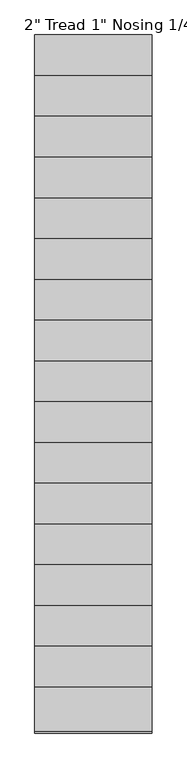
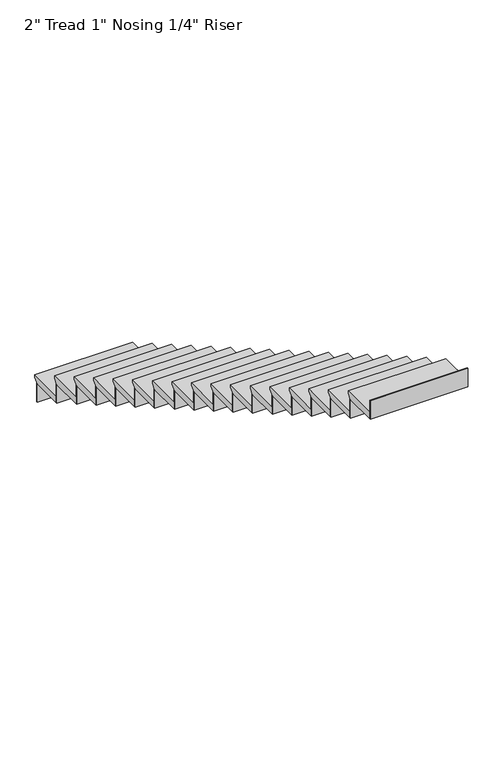
"""IFC4 building model written with IfcOpenShell, lengths in millimetres: stair flight geometry."""

from ifc_helpers import new_model, si_unit, frame, origin, place, context, project, spatial, polyline, outline, extrude, source, transform, mapped, element, save


def stair_flight_47155580(model_context):
    return source(origin(), model_context, "Body", "SweptSolid", [
        extrude(outline(polyline([(5740.7076853, 1022.35), (6020.1076853, 1022.35), (6020.1076853, 1003.3), (5994.7076853, 977.9), (5994.7076853, 971.55), (5740.7076853, 971.55), (5740.7076853, 1022.35)])), frame((-6854.5155596, 0.0, 0.0), z_axis=(1.0, 0.0, 0.0), x_axis=(0.0, 1.0, 0.0)), (0.0, 0.0, 1.0), 731.52),
        extrude(outline(polyline([(-6854.5155596, 5988.3576853), (-6854.5155596, 5994.7076853), (-6122.9955596, 5994.7076853), (-6122.9955596, 5988.3576853), (-6854.5155596, 5988.3576853)])), frame((0.0, 0.0, 825.5), z_axis=(0.0, 0.0, 1.0), x_axis=(1.0, 0.0, 0.0)), (0.0, 0.0, 1.0), 146.05),
        extrude(outline(polyline([(-6854.5155596, 5734.3576853), (-6854.5155596, 5740.7076853), (-6122.9955596, 5740.7076853), (-6122.9955596, 5734.3576853), (-6854.5155596, 5734.3576853)])), frame((0.0, 0.0, 971.55), z_axis=(0.0, 0.0, 1.0), x_axis=(1.0, 0.0, 0.0)), (0.0, 0.0, 1.0), 146.05),
        extrude(outline(polyline([(5486.7076853, 1168.4), (5766.1076853, 1168.4), (5766.1076853, 1149.35), (5740.7076853, 1123.95), (5740.7076853, 1117.6), (5486.7076853, 1117.6), (5486.7076853, 1168.4)])), frame((-6854.5155596, 0.0, 0.0), z_axis=(1.0, 0.0, 0.0), x_axis=(0.0, 1.0, 0.0)), (0.0, 0.0, 1.0), 731.52),
        extrude(outline(polyline([(-6854.5155596, 5480.3576853), (-6854.5155596, 5486.7076853), (-6122.9955596, 5486.7076853), (-6122.9955596, 5480.3576853), (-6854.5155596, 5480.3576853)])), frame((0.0, 0.0, 1117.6), z_axis=(0.0, 0.0, 1.0), x_axis=(1.0, 0.0, 0.0)), (0.0, 0.0, 1.0), 146.05),
        extrude(outline(polyline([(5232.7076853, 1314.45), (5512.1076853, 1314.45), (5512.1076853, 1295.4), (5486.7076853, 1270.0), (5486.7076853, 1263.65), (5232.7076853, 1263.65), (5232.7076853, 1314.45)])), frame((-6854.5155596, 0.0, 0.0), z_axis=(1.0, 0.0, 0.0), x_axis=(0.0, 1.0, 0.0)), (0.0, 0.0, 1.0), 731.52),
        extrude(outline(polyline([(-6854.5155596, 5226.3576853), (-6854.5155596, 5232.7076853), (-6122.9955596, 5232.7076853), (-6122.9955596, 5226.3576853), (-6854.5155596, 5226.3576853)])), frame((0.0, 0.0, 1263.65), z_axis=(0.0, 0.0, 1.0), x_axis=(1.0, 0.0, 0.0)), (0.0, 0.0, 1.0), 146.05),
        extrude(outline(polyline([(4978.7076853, 1460.5), (5258.1076853, 1460.5), (5258.1076853, 1441.45), (5232.7076853, 1416.05), (5232.7076853, 1409.7), (4978.7076853, 1409.7), (4978.7076853, 1460.5)])), frame((-6854.5155596, 0.0, 0.0), z_axis=(1.0, 0.0, 0.0), x_axis=(0.0, 1.0, 0.0)), (0.0, 0.0, 1.0), 731.52),
        extrude(outline(polyline([(-6854.5155596, 4972.3576853), (-6854.5155596, 4978.7076853), (-6122.9955596, 4978.7076853), (-6122.9955596, 4972.3576853), (-6854.5155596, 4972.3576853)])), frame((0.0, 0.0, 1409.7), z_axis=(0.0, 0.0, 1.0), x_axis=(1.0, 0.0, 0.0)), (0.0, 0.0, 1.0), 146.05),
        extrude(outline(polyline([(4724.7076853, 1606.55), (5004.1076853, 1606.55), (5004.1076853, 1587.5), (4978.7076853, 1562.1), (4978.7076853, 1555.75), (4724.7076853, 1555.75), (4724.7076853, 1606.55)])), frame((-6854.5155596, 0.0, 0.0), z_axis=(1.0, 0.0, 0.0), x_axis=(0.0, 1.0, 0.0)), (0.0, 0.0, 1.0), 731.52),
        extrude(outline(polyline([(-6854.5155596, 4718.3576853), (-6854.5155596, 4724.7076853), (-6122.9955596, 4724.7076853), (-6122.9955596, 4718.3576853), (-6854.5155596, 4718.3576853)])), frame((0.0, 0.0, 1555.75), z_axis=(0.0, 0.0, 1.0), x_axis=(1.0, 0.0, 0.0)), (0.0, 0.0, 1.0), 146.05),
        extrude(outline(polyline([(4470.7076853, 1752.6), (4750.1076853, 1752.6), (4750.1076853, 1733.55), (4724.7076853, 1708.15), (4724.7076853, 1701.8), (4470.7076853, 1701.8), (4470.7076853, 1752.6)])), frame((-6854.5155596, 0.0, 0.0), z_axis=(1.0, 0.0, 0.0), x_axis=(0.0, 1.0, 0.0)), (0.0, 0.0, 1.0), 731.52),
        extrude(outline(polyline([(-6854.5155596, 4464.3576853), (-6854.5155596, 4470.7076853), (-6122.9955596, 4470.7076853), (-6122.9955596, 4464.3576853), (-6854.5155596, 4464.3576853)])), frame((0.0, 0.0, 1701.8), z_axis=(0.0, 0.0, 1.0), x_axis=(1.0, 0.0, 0.0)), (0.0, 0.0, 1.0), 146.05),
        extrude(outline(polyline([(4216.7076853, 1898.65), (4496.1076853, 1898.65), (4496.1076853, 1879.6), (4470.7076853, 1854.2), (4470.7076853, 1847.85), (4216.7076853, 1847.85), (4216.7076853, 1898.65)])), frame((-6854.5155596, 0.0, 0.0), z_axis=(1.0, 0.0, 0.0), x_axis=(0.0, 1.0, 0.0)), (0.0, 0.0, 1.0), 731.52),
        extrude(outline(polyline([(-6854.5155596, 4210.3576853), (-6854.5155596, 4216.7076853), (-6122.9955596, 4216.7076853), (-6122.9955596, 4210.3576853), (-6854.5155596, 4210.3576853)])), frame((0.0, 0.0, 1847.85), z_axis=(0.0, 0.0, 1.0), x_axis=(1.0, 0.0, 0.0)), (0.0, 0.0, 1.0), 146.05),
        extrude(outline(polyline([(3962.7076853, 2044.7), (4242.1076853, 2044.7), (4242.1076853, 2025.65), (4216.7076853, 2000.25), (4216.7076853, 1993.9), (3962.7076853, 1993.9), (3962.7076853, 2044.7)])), frame((-6854.5155596, 0.0, 0.0), z_axis=(1.0, 0.0, 0.0), x_axis=(0.0, 1.0, 0.0)), (0.0, 0.0, 1.0), 731.52),
        extrude(outline(polyline([(-6854.5155596, 3956.3576853), (-6854.5155596, 3962.7076853), (-6122.9955596, 3962.7076853), (-6122.9955596, 3956.3576853), (-6854.5155596, 3956.3576853)])), frame((0.0, 0.0, 1993.9), z_axis=(0.0, 0.0, 1.0), x_axis=(1.0, 0.0, 0.0)), (0.0, 0.0, 1.0), 146.05),
        extrude(outline(polyline([(3708.7076853, 2190.75), (3988.1076853, 2190.75), (3988.1076853, 2171.7), (3962.7076853, 2146.3), (3962.7076853, 2139.95), (3708.7076853, 2139.95), (3708.7076853, 2190.75)])), frame((-6854.5155596, 0.0, 0.0), z_axis=(1.0, 0.0, 0.0), x_axis=(0.0, 1.0, 0.0)), (0.0, 0.0, 1.0), 731.52),
        extrude(outline(polyline([(-6854.5155596, 3702.3576853), (-6854.5155596, 3708.7076853), (-6122.9955596, 3708.7076853), (-6122.9955596, 3702.3576853), (-6854.5155596, 3702.3576853)])), frame((0.0, 0.0, 2139.95), z_axis=(0.0, 0.0, 1.0), x_axis=(1.0, 0.0, 0.0)), (0.0, 0.0, 1.0), 146.05),
        extrude(outline(polyline([(3454.7076853, 2336.8), (3734.1076853, 2336.8), (3734.1076853, 2317.75), (3708.7076853, 2292.35), (3708.7076853, 2286.0), (3454.7076853, 2286.0), (3454.7076853, 2336.8)])), frame((-6854.5155596, 0.0, 0.0), z_axis=(1.0, 0.0, 0.0), x_axis=(0.0, 1.0, 0.0)), (0.0, 0.0, 1.0), 731.52),
        extrude(outline(polyline([(-6854.5155596, 3448.3576853), (-6854.5155596, 3454.7076853), (-6122.9955596, 3454.7076853), (-6122.9955596, 3448.3576853), (-6854.5155596, 3448.3576853)])), frame((0.0, 0.0, 2286.0), z_axis=(0.0, 0.0, 1.0), x_axis=(1.0, 0.0, 0.0)), (0.0, 0.0, 1.0), 146.05),
        extrude(outline(polyline([(3200.7076853, 2482.85), (3480.1076853, 2482.85), (3480.1076853, 2463.8), (3454.7076853, 2438.4), (3454.7076853, 2432.05), (3200.7076853, 2432.05), (3200.7076853, 2482.85)])), frame((-6854.5155596, 0.0, 0.0), z_axis=(1.0, 0.0, 0.0), x_axis=(0.0, 1.0, 0.0)), (0.0, 0.0, 1.0), 731.52),
        extrude(outline(polyline([(-6854.5155596, 3194.3576853), (-6854.5155596, 3200.7076853), (-6122.9955596, 3200.7076853), (-6122.9955596, 3194.3576853), (-6854.5155596, 3194.3576853)])), frame((0.0, 0.0, 2432.05), z_axis=(0.0, 0.0, 1.0), x_axis=(1.0, 0.0, 0.0)), (0.0, 0.0, 1.0), 146.05),
        extrude(outline(polyline([(2946.7076853, 2628.9), (3226.1076853, 2628.9), (3226.1076853, 2609.85), (3200.7076853, 2584.45), (3200.7076853, 2578.1), (2946.7076853, 2578.1), (2946.7076853, 2628.9)])), frame((-6854.5155596, 0.0, 0.0), z_axis=(1.0, 0.0, 0.0), x_axis=(0.0, 1.0, 0.0)), (0.0, 0.0, 1.0), 731.52),
        extrude(outline(polyline([(-6854.5155596, 2940.3576853), (-6854.5155596, 2946.7076853), (-6122.9955596, 2946.7076853), (-6122.9955596, 2940.3576853), (-6854.5155596, 2940.3576853)])), frame((0.0, 0.0, 2578.1), z_axis=(0.0, 0.0, 1.0), x_axis=(1.0, 0.0, 0.0)), (0.0, 0.0, 1.0), 146.05),
        extrude(outline(polyline([(2692.7076853, 2774.95), (2972.1076853, 2774.95), (2972.1076853, 2755.9), (2946.7076853, 2730.5), (2946.7076853, 2724.15), (2692.7076853, 2724.15), (2692.7076853, 2774.95)])), frame((-6854.5155596, 0.0, 0.0), z_axis=(1.0, 0.0, 0.0), x_axis=(0.0, 1.0, 0.0)), (0.0, 0.0, 1.0), 731.52),
        extrude(outline(polyline([(-6854.5155596, 2686.3576853), (-6854.5155596, 2692.7076853), (-6122.9955596, 2692.7076853), (-6122.9955596, 2686.3576853), (-6854.5155596, 2686.3576853)])), frame((0.0, 0.0, 2724.15), z_axis=(0.0, 0.0, 1.0), x_axis=(1.0, 0.0, 0.0)), (0.0, 0.0, 1.0), 146.05),
        extrude(outline(polyline([(2438.7076853, 2921.0), (2718.1076853, 2921.0), (2718.1076853, 2901.95), (2692.7076853, 2876.55), (2692.7076853, 2870.2), (2438.7076853, 2870.2), (2438.7076853, 2921.0)])), frame((-6854.5155596, 0.0, 0.0), z_axis=(1.0, 0.0, 0.0), x_axis=(0.0, 1.0, 0.0)), (0.0, 0.0, 1.0), 731.52),
        extrude(outline(polyline([(-6854.5155596, 2432.3576853), (-6854.5155596, 2438.7076853), (-6122.9955596, 2438.7076853), (-6122.9955596, 2432.3576853), (-6854.5155596, 2432.3576853)])), frame((0.0, 0.0, 2870.2), z_axis=(0.0, 0.0, 1.0), x_axis=(1.0, 0.0, 0.0)), (0.0, 0.0, 1.0), 146.05),
        extrude(outline(polyline([(2184.7076853, 3067.05), (2464.1076853, 3067.05), (2464.1076853, 3048.0), (2438.7076853, 3022.6), (2438.7076853, 3016.25), (2184.7076853, 3016.25), (2184.7076853, 3067.05)])), frame((-6854.5155596, 0.0, 0.0), z_axis=(1.0, 0.0, 0.0), x_axis=(0.0, 1.0, 0.0)), (0.0, 0.0, 1.0), 731.52),
        extrude(outline(polyline([(-6854.5155596, 2178.3576853), (-6854.5155596, 2184.7076853), (-6122.9955596, 2184.7076853), (-6122.9955596, 2178.3576853), (-6854.5155596, 2178.3576853)])), frame((0.0, 0.0, 3016.25), z_axis=(0.0, 0.0, 1.0), x_axis=(1.0, 0.0, 0.0)), (0.0, 0.0, 1.0), 146.05),
        extrude(outline(polyline([(1930.7076853, 3213.1), (2210.1076853, 3213.1), (2210.1076853, 3194.05), (2184.7076853, 3168.65), (2184.7076853, 3162.3), (1930.7076853, 3162.3), (1930.7076853, 3213.1)])), frame((-6854.5155596, 0.0, 0.0), z_axis=(1.0, 0.0, 0.0), x_axis=(0.0, 1.0, 0.0)), (0.0, 0.0, 1.0), 731.52),
        extrude(outline(polyline([(-6854.5155596, 1924.3576853), (-6854.5155596, 1930.7076853), (-6122.9955596, 1930.7076853), (-6122.9955596, 1924.3576853), (-6854.5155596, 1924.3576853)])), frame((0.0, 0.0, 3162.3), z_axis=(0.0, 0.0, 1.0), x_axis=(1.0, 0.0, 0.0)), (0.0, 0.0, 1.0), 146.05),
        extrude(outline(polyline([(-6854.5155596, 1670.3576853), (-6854.5155596, 1676.7076853), (-6122.9955596, 1676.7076853), (-6122.9955596, 1670.3576853), (-6854.5155596, 1670.3576853)])), frame((0.0, 0.0, 3308.35), z_axis=(0.0, 0.0, 1.0), x_axis=(1.0, 0.0, 0.0)), (0.0, 0.0, 1.0), 146.05),
        extrude(outline(polyline([(1676.7076853, 3359.15), (1956.1076853, 3359.15), (1956.1076853, 3340.1), (1930.7076853, 3314.7), (1930.7076853, 3308.35), (1676.7076853, 3308.35), (1676.7076853, 3359.15)])), frame((-6854.5155596, 0.0, 0.0), z_axis=(1.0, 0.0, 0.0), x_axis=(0.0, 1.0, 0.0)), (0.0, 0.0, 1.0), 731.52),
    ])


if __name__ == "__main__":
    model = new_model("IFC4")
    model_context = context("Model", 3, world=origin())
    ifc_project = project(units=[si_unit("LENGTHUNIT", "METRE", prefix="MILLI")], contexts=[model_context])
    site = spatial("IfcSite", under=ifc_project)
    building = spatial("IfcBuilding", under=site)
    placement = place(None, origin())
    stair_flight_shape = stair_flight_47155580(model_context)
    element("IfcStairFlight", 1, ObjectType="2\" Tread 1\" Nosing 1/4\" Riser", at=placement, inside=building, context=model_context, shape_type="MappedRepresentation", body=[
        mapped(stair_flight_shape, transform((0.0, 0.0, 0.0), x_axis=(1.0, 0.0, 0.0), y_axis=(0.0, 1.0, 0.0), z_axis=(0.0, 0.0, 1.0))),
    ])
    save(model, "model.ifc")
